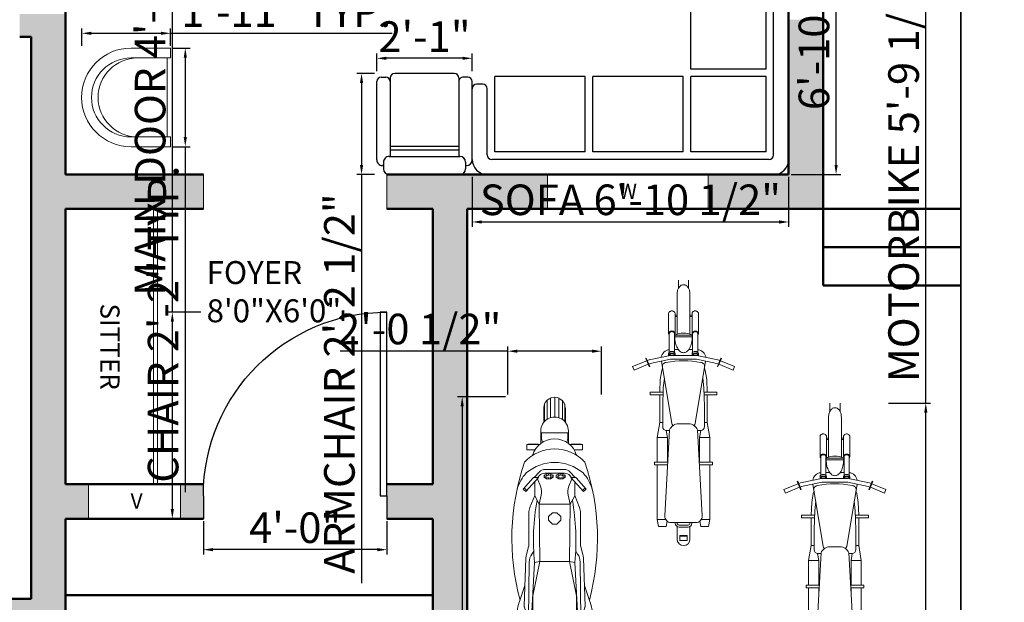
# Model space of a CAD drawing. Units: inches. Extents: x 3354 to 4308, y 1668 to 2317.
# Tile 4 of 11: x 3534 to 3792, y 1807 to 1960. Entities that reach past the tile are written whole.
import ezdxf

# ---------------------------------------------------------------- set-up
doc = ezdxf.new("R2010")
doc.units = ezdxf.units.IN
for name, color, linetype, lineweight in [('A-ANNO-DIMS', 2, 'Continuous', 18), ('A-ANNO-TEXT', 7, 'Continuous', 18), ('A-AREA-IDEN', 3, 'Continuous', 18), ('A-DOOR', 3, 'Continuous', 25), ('A-EQPM', 9, 'Continuous', 18), ('A-FURN', 8, 'Continuous', 18), ('A-GLAZ', 4, 'Continuous', 18), ('A-WALL', 7, 'Continuous', 50), ('A-WALL-PATT', 8, 'Continuous', 13), ('C-PROP', 1, 'Continuous', 35)]:
    doc.layers.add(name, color=color, linetype=linetype, lineweight=lineweight)
doc.layers.add('M40-KOLTUKSUNGERI', color=136, linetype='Continuous')
doc.layers.add('wood', color=26, linetype='Continuous')
doc.styles.get("Standard").update_dxf_attribs({"font": 'arial.ttf'})
doc.dimstyles.new('ISO-25', dxfattribs={"dimtxt": 8, "dimasz": 2.5, "dimexe": 1.25, "dimexo": 0.625, "dimtad": 1, "dimdec": 1, "dimlunit": 3, "dimtxsty": 'Standard', "dimcen": 2.5, "dimadec": 0, "dimazin": 0, "dimtfac": 1, "dimtdec": 1, "dimtmove": 0, "dimatfit": 3, "dimfxl": 1, "dimarcsym": 0})

# ---------------------------------------------------------------- blocks, each defined once
blk = doc.blocks.new('DOOR')
for p, q in [((0, 6), (0, 0)), ((48, 6), (48, 0))]:
    blk.add_line(p, q)
blk.add_lwpolyline([(0, 6), (0, 54), (1.75, 54), (1.75, 6)], close=True)
blk.add_arc((0, 6), 48, 0, 90)
blk = doc.blocks.new('12PSTG07')
at = {"color": 0, "linetype": 'ByBlock'}
for p, q in [((0, 15), (-12, 15)), ((0, 12), (0, 15)), ((-12, 12), (0, 12)), ((-1, -12), (-1, 12)), ((-12, -12), (0, -12)), ((0, -12), (0, -15)), ((0, -15), (-12, -15))]:
    blk.add_line(p, q, dxfattribs=at)
for centre, radius in [((-12, 0), 15), ((-12, 0), 12), ((-10, 0), 12)]:
    blk.add_arc(centre, radius, 90, 270, dxfattribs=at)
blk = doc.blocks.new('BIKE')
for p, q in [((34846.04, 15170.34), (34846.04, 15168.87)), ((34847.86, 15170.34), (34847.86, 15168.87)), ((34845.81, 15167.86), (34845.81, 15160.7)), ((34845.81, 15167.86), (34845.81, 15160.7)), ((34848.09, 15167.86), (34848.09, 15160.7)), ((34844.29, 15164.4), (34844.29, 15160.81)), ((34845.43, 15164.4), (34845.43, 15160.81)), ((34845.43, 15164.1), (34845.81, 15164.1)), ((34845.43, 15163.85), (34845.81, 15163.85)), ((34848.47, 15164.1), (34848.09, 15164.1)), ((34848.47, 15163.85), (34848.09, 15163.85)), ((34848.47, 15164.4), (34848.47, 15160.81)), ((34849.61, 15164.4), (34849.61, 15160.81)), ((34844.41, 15160.81), (34844.41, 15157.43)), ((34845.32, 15160.81), (34845.32, 15157.43)), ((34848.51, 15160.53), (34845.39, 15160.53)), ((34845.39, 15160.23), (34845.39, 15160.53)), ((34845.39, 15160.23), (34845.39, 15160.53)), ((34848.51, 15160.23), (34845.39, 15160.23)), ((34848.51, 15160.23), (34848.51, 15160.53)), ((34848.58, 15160.81), (34848.58, 15157.43)), ((34849.5, 15160.81), (34849.5, 15157.43)), ((34845.32, 15157.92), (34846.04, 15157.92)), ((34848.58, 15157.92), (34847.87, 15157.92)), ((34837.84, 15154.89), (34840.37, 15155.93)), ((34840.19, 15156.35), (34840.3, 15156.39)), ((34840.19, 15156.35), (34840.8, 15154.88)), ((34840.3, 15156.39), (34840.9, 15154.92)), ((34840.47, 15155.97), (34840.8, 15156.11)), ((34840.8, 15156.11), (34844.56, 15156.88)), ((34841, 15155.45), (34844.63, 15156.2)), ((34844.86, 15144.72), (34843.01, 15155.87)), ((34844.29, 15156.87), (34844.29, 15157.17)), ((34844.41, 15156.87), (34844.41, 15156.85)), ((34844.56, 15156.88), (34846.95, 15156.88)), ((34844.63, 15156.2), (34846.95, 15156.2)), ((34845.43, 15156.87), (34845.43, 15157.17)), ((34849.34, 15156.88), (34846.95, 15156.88)), ((34849.27, 15156.2), (34846.95, 15156.2)), ((34848.47, 15156.87), (34848.47, 15157.17)), ((34849.05, 15144.72), (34850.89, 15155.87)), ((34852.9, 15155.45), (34849.27, 15156.2)), ((34853.1, 15156.11), (34849.34, 15156.88)), ((34849.5, 15156.87), (34849.5, 15156.85)), ((34849.61, 15156.87), (34849.61, 15157.17)), ((34853.6, 15156.39), (34853, 15154.92)), ((34853.71, 15156.35), (34853.1, 15154.88)), ((34853.43, 15155.97), (34853.1, 15156.11)), ((34856.07, 15154.89), (34853.54, 15155.93)), ((34853.71, 15156.35), (34853.6, 15156.39)), ((34837.84, 15154.89), (34838.1, 15154.26)), ((34838.1, 15154.26), (34840.63, 15155.3)), ((34840.73, 15155.34), (34841, 15155.45)), ((34840.8, 15154.88), (34840.9, 15154.92)), ((34842.8, 15152.59), (34843.06, 15154.2)), ((34843.06, 15154.2), (34843.22, 15154.58)), ((34850.84, 15154.2), (34850.68, 15154.58)), ((34851.1, 15152.59), (34850.84, 15154.2)), ((34853.17, 15155.34), (34852.9, 15155.45)), ((34853.1, 15154.88), (34853, 15154.92)), ((34855.81, 15154.26), (34853.28, 15155.3)), ((34856.07, 15154.89), (34855.81, 15154.26)), ((34842.7, 15150.31), (34842.8, 15152.59)), ((34843.33, 15151.09), (34843.52, 15152.8)), ((34850.57, 15151.09), (34850.38, 15152.8)), ((34851.2, 15150.31), (34851.1, 15152.59)), ((34843.23, 15147.75), (34843.33, 15151.09)), ((34850.67, 15147.75), (34850.57, 15151.09)), ((34840.97, 15150.31), (34843.3, 15150.31)), ((34840.97, 15149.81), (34840.97, 15150.31)), ((34843.29, 15149.81), (34840.97, 15149.81)), ((34842.7, 15144.87), (34842.7, 15149.81)), ((34852.93, 15150.31), (34850.6, 15150.31)), ((34850.61, 15149.81), (34852.93, 15149.81)), ((34851.2, 15144.87), (34851.2, 15149.81)), ((34852.93, 15149.81), (34852.93, 15150.31)), ((34843.23, 15144.15), (34843.23, 15147.75)), ((34850.67, 15144.15), (34850.67, 15147.75)), ((34842.7, 15144.87), (34842.25, 15142.19)), ((34842.7, 15144.87), (34843.23, 15144.87)), ((34844.46, 15143.56), (34843.6, 15128.2)), ((34847.85, 15144.64), (34846.06, 15144.64)), ((34849.44, 15143.56), (34850.3, 15128.2)), ((34851.2, 15144.87), (34850.67, 15144.87)), ((34851.2, 15144.87), (34851.65, 15142.19)), ((34842.25, 15142.19), (34844.07, 15142.19)), ((34842.25, 15137.82), (34842.25, 15142.19)), ((34843.85, 15143.46), (34844.07, 15142.19)), ((34843.91, 15143.46), (34844.46, 15143.46)), ((34844.07, 15137.82), (34844.07, 15142.19)), ((34849.99, 15143.46), (34849.44, 15143.46)), ((34850.05, 15143.46), (34849.83, 15142.19)), ((34851.65, 15142.19), (34849.83, 15142.19)), ((34849.83, 15137.82), (34849.83, 15142.19)), ((34851.65, 15137.82), (34851.65, 15142.19)), ((34841.79, 15137.82), (34844.14, 15137.82)), ((34841.79, 15137.33), (34841.79, 15137.82)), ((34844.11, 15137.33), (34841.79, 15137.33)), ((34842.25, 15127.57), (34842.25, 15137.33)), ((34844.07, 15136.55), (34844.07, 15137.33)), ((34852.11, 15137.82), (34849.76, 15137.82)), ((34849.79, 15137.33), (34852.11, 15137.33)), ((34849.83, 15136.55), (34849.83, 15137.33)), ((34851.65, 15127.57), (34851.65, 15137.33)), ((34852.11, 15137.33), (34852.11, 15137.82)), ((34842.25, 15127.57), (34843.75, 15127.57)), ((34842.25, 15127.57), (34842.48, 15126.27)), ((34842.48, 15126.27), (34843.84, 15126.27)), ((34844.02, 15127.25), (34843.84, 15126.27)), ((34849.16, 15126.99), (34844.74, 15126.99)), ((34845.47, 15126.99), (34845.47, 15126.88)), ((34845.81, 15126.99), (34845.81, 15126.88)), ((34845.81, 15126.29), (34845.81, 15124.03)), ((34847.75, 15126.54), (34846.15, 15126.54)), ((34847.75, 15126.2), (34846.15, 15126.2)), ((34848.09, 15126.99), (34848.09, 15126.88)), ((34848.09, 15126.29), (34848.09, 15124.03)), ((34848.43, 15126.99), (34848.43, 15126.88)), ((34849.89, 15127.25), (34850.06, 15126.27)), ((34851.43, 15126.27), (34850.06, 15126.27)), ((34851.65, 15127.57), (34850.15, 15127.57)), ((34851.65, 15127.57), (34851.43, 15126.27)), ((34846.29, 15123.82), (34846.29, 15124.66)), ((34846.29, 15124.66), (34847.61, 15124.66)), ((34846.29, 15124.55), (34847.61, 15124.55)), ((34847.61, 15124.66), (34847.61, 15123.82)), ((34847.61, 15123.82), (34846.29, 15123.82))]:
    blk.add_line(p, q)
for points in [[(34845.81, 15167.86, -0.068977), (34845.9, 15168.53, -0.081012), (34846.15, 15169.05, -0.107014), (34846.54, 15169.42, -0.137239), (34846.95, 15169.53, -0.137239), (34847.36, 15169.42, -0.107014), (34847.76, 15169.05, -0.081012), (34848, 15168.53, -0.068977), (34848.09, 15167.86, -0.068977)], [(34845.43, 15164.4, 0.125099), (34845.39, 15164.56, 0.105827), (34845.27, 15164.71, 0.086577), (34845.09, 15164.8, 0.0766), (34844.86, 15164.84, 0.0766), (34844.64, 15164.8, 0.086577), (34844.46, 15164.71, 0.105827), (34844.33, 15164.56, 0.125099), (34844.29, 15164.4, 0.125099)], [(34848.47, 15164.4, -0.125099), (34848.51, 15164.56, -0.105827), (34848.64, 15164.71, -0.086577), (34848.82, 15164.8, -0.0766), (34849.04, 15164.84, -0.0766), (34849.26, 15164.8, -0.086577), (34849.44, 15164.71, -0.105827), (34849.57, 15164.56, -0.125099), (34849.61, 15164.4, -0.125099)], [(34845.32, 15160.55, 0.067261), (34845.39, 15160.65, 0.125099), (34845.43, 15160.81, 0.125099), (34845.39, 15160.97, 0.105827), (34845.27, 15161.12, 0.086577), (34845.09, 15161.21, 0.0766), (34844.86, 15161.25, 0.0766), (34844.64, 15161.21, 0.086577), (34844.46, 15161.12, 0.105827), (34844.33, 15160.97, 0.125099), (34844.29, 15160.81, 0.125099)], [(34845.32, 15160.81, 0.125099), (34845.29, 15160.92, 0.105827), (34845.2, 15161.03, 0.086577), (34845.05, 15161.1, 0.0766), (34844.86, 15161.13, 0.0766), (34844.67, 15161.1, 0.086577), (34844.53, 15161.03, 0.105827), (34844.43, 15160.92, 0.125099), (34844.41, 15160.81, 0.125099)], [(34848.58, 15160.55, -0.067261), (34848.51, 15160.65, -0.125099), (34848.47, 15160.81, -0.125099), (34848.51, 15160.97, -0.105827), (34848.64, 15161.12, -0.086577), (34848.82, 15161.21, -0.0766), (34849.04, 15161.25, -0.0766), (34849.26, 15161.21, -0.086577), (34849.44, 15161.12, -0.105827), (34849.57, 15160.97, -0.125099), (34849.61, 15160.81, -0.125099)], [(34848.58, 15160.81, -0.125099), (34848.61, 15160.92, -0.105827), (34848.71, 15161.03, -0.086577), (34848.85, 15161.1, -0.0766), (34849.04, 15161.13, -0.0766), (34849.23, 15161.1, -0.086577), (34849.37, 15161.03, -0.105827), (34849.47, 15160.92, -0.125099), (34849.5, 15160.81, -0.125099)], [(34844.29, 15160.81, 0.125099), (34844.33, 15160.65, 0.067261), (34844.41, 15160.55, 0.086577)], [(34846.95, 15157.37, -0.163989), (34846.41, 15157.55, -0.105862), (34845.85, 15158.21, -0.069323), (34845.52, 15159.08, -0.055531), (34845.39, 15160.23, -0.055531)], [(34848.51, 15160.23, -0.055531), (34848.38, 15159.08, -0.069323), (34848.06, 15158.21, -0.105862), (34847.49, 15157.55, -0.163989), (34846.95, 15157.37, -0.163989)], [(34849.61, 15160.81, -0.125099), (34849.57, 15160.65, -0.067261), (34849.5, 15160.55, -0.086577)], [(34845.43, 15157.17, 0.125099), (34845.39, 15157.33, 0.105827), (34845.27, 15157.48, 0.086577), (34845.09, 15157.57, 0.0766), (34844.86, 15157.6, 0.0766), (34844.64, 15157.57, 0.086577), (34844.46, 15157.48, 0.105827), (34844.33, 15157.33, 0.125099), (34844.29, 15157.17, 0.125099)], [(34848.47, 15157.17, -0.125099), (34848.51, 15157.33, -0.105827), (34848.64, 15157.48, -0.086577), (34848.82, 15157.57, -0.0766), (34849.04, 15157.6, -0.0766), (34849.26, 15157.57, -0.086577), (34849.44, 15157.48, -0.105827), (34849.57, 15157.33, -0.125099), (34849.61, 15157.17, -0.125099)], [(34845.43, 15156.88, 0.117252), (34845.39, 15157.03, 0.105827), (34845.27, 15157.18, 0.086577), (34845.09, 15157.27, 0.0766), (34844.86, 15157.31, 0.0766), (34844.64, 15157.27, 0.086577), (34844.46, 15157.18, 0.105827), (34844.33, 15157.03, 0.125099), (34844.29, 15156.87, 0.125099)], [(34844.29, 15156.87, 0.032819), (34844.3, 15156.83, 0.067261)], [(34845.32, 15156.88, 0.113202), (34845.29, 15156.98, 0.105827), (34845.2, 15157.09, 0.086577), (34845.05, 15157.16, 0.0766), (34844.86, 15157.19, 0.0766), (34844.67, 15157.16, 0.086577), (34844.53, 15157.09, 0.105827), (34844.43, 15156.98, 0.125099), (34844.41, 15156.87, 0.125099)], [(34848.47, 15156.88, -0.117252), (34848.51, 15157.03, -0.105827), (34848.64, 15157.18, -0.086577), (34848.82, 15157.27, -0.0766), (34849.04, 15157.31, -0.0766), (34849.26, 15157.27, -0.086577), (34849.44, 15157.18, -0.105827), (34849.57, 15157.03, -0.125099), (34849.61, 15156.87, -0.125099)], [(34848.58, 15156.88, -0.113202), (34848.61, 15156.98, -0.105827), (34848.71, 15157.09, -0.086577), (34848.85, 15157.16, -0.0766), (34849.04, 15157.19, -0.0766), (34849.23, 15157.16, -0.086577), (34849.37, 15157.09, -0.105827), (34849.47, 15156.98, -0.125099), (34849.5, 15156.87, -0.125099)], [(34849.61, 15156.87, -0.032819), (34849.61, 15156.83, -0.067261)]]:
    blk.add_lwpolyline(points, format="xyb")
for centre, radius, start, end in [((34846.95, 15157.24), 3.64, 64.5882, 115.4118), ((34844.55, 15156.32), 1.59, 95.2207, 171.678), ((34849.35, 15156.32), 1.59, 8.322, 84.7793), ((34846.95, 15140.12), 15.79, 78.7129, 101.2871), ((34843.86, 15154.92), 0.684, 90, 189.3898), ((34850.04, 15154.92), 0.684, 350.6102, 90), ((34843.91, 15144.15), 0.684, 180, 270), ((34846, 15143), 1.64, 88.1125, 159.9264), ((34845.53, 15144.83), 0.684, 189.3898, 226.4877), ((34847.9, 15143), 1.64, 20.0736, 91.8875), ((34848.37, 15144.83), 0.684, 313.5123, 350.6102), ((34849.99, 15144.15), 0.684, 270, 0), ((34844.74, 15128.13), 1.14, 176.7865, 270), ((34849.16, 15128.13), 1.14, 270, 3.2135), ((34846.15, 15126.88), 0.684, 180, 270), ((34846.15, 15126.88), 0.342, 180, 270), ((34847.75, 15126.88), 0.684, 270, 0), ((34847.75, 15126.88), 0.342, 270, 0), ((34846.95, 15124.03), 1.14, 180, 0)]:
    blk.add_arc(centre, radius, start, end)
blk = doc.blocks.new('1 bike')
for p, q in [((-13.2, 41.5), (-13.2, 35.26)), ((-12.29, 42.13), (-12.29, 35.26)), ((-11.19, 35.26), (-11.19, 42.36)), ((-10.09, 42.17), (-10.09, 35.26)), ((-9.19, 41.55), (-9.19, 35.26)), ((-14.01, 39.55), (-14.01, 35.26)), ((-13.81, 35.26), (-13.81, 40.5)), ((-8.57, 35.26), (-8.57, 40.59)), ((-8.38, 39.55), (-8.38, 35.26)), ((-17.37, 30.6), (-16.62, 34.32)), ((-14.57, 34.95), (-15.85, 34.95)), ((-7.36, 33.82), (-15.02, 33.82)), ((-14.78, 35.24), (-14.17, 34.43)), ((-14.78, 35.24), (-7.6, 35.24)), ((-8.21, 34.43), (-14.17, 34.43)), ((-7.6, 35.24), (-8.21, 34.43)), ((-7.81, 34.95), (-6.53, 34.95)), ((-5.01, 30.6), (-5.76, 34.32)), ((-21.27, 32.95), (-21.54, 32.62)), ((-21.54, 32.62), (-21.28, 21.37)), ((-18.78, 32.95), (-21.27, 32.95)), ((-18.78, 32.95), (-18.43, 32.54)), ((-18.43, 32.54), (-18.57, 30.5)), ((-18.18, 30.5), (-18.46, 32.12)), ((-16.53, 30.42), (-15.78, 33.23)), ((-5.85, 30.42), (-6.6, 33.23)), ((-4.2, 30.5), (-3.92, 32.12)), ((-3.61, 32.95), (-3.95, 32.54)), ((-3.95, 32.54), (-3.81, 30.5)), ((-3.61, 32.95), (-1.11, 32.95)), ((-1.11, 32.95), (-0.84, 32.62)), ((-0.84, 32.62), (-1.1, 21.37)), ((-20.57, 28.93), (-20.57, 30.49)), ((-20.57, 30.49), (-16.95, 30.49)), ((-16.95, 28.93), (-20.57, 28.93)), ((-20.22, 30.58), (-17.31, 30.58)), ((-18.58, 28.93), (-18.58, 23.76)), ((-17.89, 28.92), (-17.63, 27.46)), ((-17.5, 28.92), (-17.66, 26.86)), ((-17.37, 30.5), (-17.37, 30.6)), ((-16.53, 30.42), (-17.37, 30.55)), ((-17.37, 30.55), (-17.37, 30.5)), ((-16.95, 30.49), (-16.95, 28.93)), ((-16.04, 27.32), (-16.53, 30.42)), ((-5.85, 30.42), (-16.5, 30.42)), ((-6.34, 27.32), (-5.85, 30.42)), ((-5.85, 30.42), (-5.01, 30.55)), ((-5.43, 30.49), (-5.43, 28.93)), ((-1.81, 30.49), (-5.43, 30.49)), ((-5.43, 28.93), (-1.81, 28.93)), ((-2.16, 30.58), (-5.08, 30.58)), ((-5.01, 30.5), (-5.01, 30.6)), ((-5.01, 30.55), (-5.01, 30.5)), ((-4.88, 28.92), (-4.72, 26.86)), ((-4.49, 28.92), (-4.75, 27.46)), ((-3.8, 28.93), (-3.8, 23.76)), ((-1.81, 28.93), (-1.81, 30.49)), ((-19.32, 21.36), (-17.66, 26.86)), ((-19.19, 21.42), (-16.04, 27.32)), ((-16.04, 27.32), (-17.98, 21.16)), ((-16.17, 25.96), (-16.89, 22.88)), ((-15.14, 27.32), (-16.17, 25.96)), ((-16.04, 27.32), (-16.08, 26.1)), ((-16.01, 27.32), (-6.34, 27.32)), ((-15.14, 24.28), (-15.14, 27.32)), ((-7.24, 27.32), (-6.21, 25.96)), ((-7.24, 24.28), (-7.24, 27.32)), ((-6.34, 27.32), (-6.31, 26.1)), ((-6.34, 27.32), (-4.4, 21.16)), ((-3.2, 21.42), (-6.34, 27.32)), ((-6.21, 25.96), (-5.5, 22.88)), ((-3.07, 21.36), (-4.72, 26.86)), ((-16.17, 21.85), (-15.14, 24.28)), ((-7.24, 24.28), (-15.11, 24.28)), ((-6.21, 21.85), (-7.24, 24.28)), ((-17.84, 6.18), (-18.02, 20.91)), ((-16.89, 22.88), (-17.14, 19.13)), ((-16.89, 19.03), (-16.17, 21.85)), ((-5.5, 19.03), (-6.21, 21.85)), ((-5.5, 22.88), (-5.24, 19.13)), ((-4.54, 6.18), (-4.37, 20.91)), ((-19.11, 17.99), (-18.54, 19.9)), ((-19.09, 20.53), (-18, 19.28)), ((-17.14, 19.13), (-16.46, 6.25)), ((-16.92, 15.02), (-16.89, 19.03)), ((-5.24, 19.13), (-5.92, 6.25)), ((-5.46, 15.02), (-5.5, 19.03)), ((-3.3, 20.53), (-4.39, 19.28)), ((-3.27, 17.99), (-3.84, 19.9)), ((-18.96, 12.28), (-20.45, 16.7)), ((-18.71, 5.16), (-19.15, 17.74)), ((-3.67, 5.16), (-3.24, 17.74)), ((-3.42, 12.28), (-1.93, 16.7)), ((-15.04, 6), (-16.92, 15.02)), ((-7.34, 6), (-5.46, 15.02)), ((-15.04, 6), (-16.46, 6.25)), ((-15.04, 6), (-16.46, 6.25)), ((-15.27, -8.98), (-15.04, 6)), ((-15.01, 6), (-7.34, 6)), ((-15.01, 6), (-7.34, 6)), ((-7.34, 6), (-5.92, 6.25)), ((-7.34, 6), (-5.92, 6.25)), ((-7.11, -8.98), (-7.34, 6)), ((-18.09, 2.47), (-18.58, 4.26)), ((-17.19, 4.06), (-16.68, 3.28)), ((-5.19, 4.06), (-5.71, 3.28)), ((-4.3, 2.47), (-3.81, 4.26)), ((-17.95, -6.66), (-17.95, 1.43)), ((-4.43, -6.66), (-4.43, 1.43)), ((-11.77, -3.74), (-12.84, -4.75)), ((-12.84, -4.75), (-12.84, -5.75)), ((-11.77, -3.74), (-10.61, -3.74)), ((-10.61, -3.74), (-9.54, -4.75)), ((-9.54, -4.75), (-9.54, -5.75)), ((-12.84, -5.75), (-11.77, -6.72)), ((-10.61, -6.72), (-11.77, -6.72)), ((-9.54, -5.75), (-10.61, -6.72)), ((-16.42, -11.25), (-17.67, -8.11)), ((-15.27, -8.98), (-16.42, -11.15)), ((-14.73, -11.31), (-15.27, -8.98)), ((-7.11, -8.98), (-15.24, -8.98)), ((-7.65, -11.31), (-7.11, -8.98)), ((-7.11, -8.98), (-5.96, -11.15)), ((-5.96, -11.25), (-4.71, -8.11)), ((-18.7, -12.25), (-19.45, -12.92)), ((-18.44, -12.54), (-19.19, -13.22)), ((-15.4, -15.97), (-18.7, -12.25)), ((-16.42, -11.15), (-16.42, -14.82)), ((-6.99, -15.97), (-3.68, -12.25)), ((-5.96, -11.15), (-5.96, -14.82)), ((-3.94, -12.54), (-3.19, -13.22)), ((-3.68, -12.25), (-2.93, -12.92)), ((-19.45, -12.92), (-16.84, -15.84)), ((-15.69, -15.57), (-14.92, -13.66)), ((-6.69, -15.57), (-7.46, -13.66)), ((-2.93, -12.92), (-5.54, -15.84)), ((-16.55, -15.97), (-15.4, -15.97)), ((-16.51, -15.99), (-15.16, -17.42)), ((-15.17, -16.45), (-15.61, -15.99)), ((-13.97, -16), (-13.29, -15.62)), ((-13.97, -16.52), (-13.97, -16)), ((-13.29, -16.91), (-13.97, -16.52)), ((-13.29, -16.1), (-13.75, -16.04)), ((-13.75, -16.36), (-13.29, -16.26)), ((-13.74, -17.07), (-8.65, -17.07)), ((-13.39, -15.74), (-13.1, -15.97)), ((-13.1, -16.42), (-13.39, -16.62)), ((-12.29, -15.62), (-13.29, -15.62)), ((-12.29, -16.91), (-13.29, -16.91)), ((-12.78, -15.91), (-12.78, -15.65)), ((-12.78, -16.49), (-12.78, -16.72)), ((-12.19, -15.74), (-12.45, -15.97)), ((-12.45, -16.42), (-12.19, -16.62)), ((-12.29, -15.62), (-11.58, -16)), ((-12.29, -16.91), (-11.58, -16.52)), ((-11.81, -16.04), (-12.26, -16.1)), ((-12.26, -16.26), (-11.81, -16.36)), ((-11.58, -16.52), (-11.58, -16)), ((-10.09, -15.62), (-10.8, -16)), ((-10.8, -16.52), (-10.8, -16)), ((-10.09, -16.91), (-10.8, -16.52)), ((-10.58, -16.04), (-10.12, -16.1)), ((-10.12, -16.26), (-10.58, -16.36)), ((-10.19, -15.74), (-9.93, -15.97)), ((-9.93, -16.42), (-10.19, -16.62)), ((-10.09, -15.62), (-9.09, -15.62)), ((-10.09, -16.91), (-9.09, -16.91)), ((-9.61, -15.91), (-9.61, -15.65)), ((-9.61, -16.49), (-9.61, -16.72)), ((-8.99, -15.74), (-9.28, -15.97)), ((-9.28, -16.42), (-8.99, -16.62)), ((-8.41, -16), (-9.09, -15.62)), ((-9.09, -16.1), (-8.64, -16.04)), ((-8.64, -16.36), (-9.09, -16.26)), ((-9.09, -16.91), (-8.41, -16.52)), ((-8.41, -16.52), (-8.41, -16)), ((-5.87, -15.99), (-7.22, -17.42)), ((-7.21, -16.45), (-6.77, -15.99)), ((-5.83, -15.97), (-6.99, -15.97)), ((-8.65, -18.04), (-13.73, -18.04)), ((-18.47, -24.58), (-18.47, -23.15)), ((-18.47, -23.15), (-16.35, -23.15)), ((-3.91, -23.15), (-6.03, -23.15)), ((-3.91, -24.58), (-3.91, -23.15)), ((-15.14, -24.58), (-18.47, -24.58)), ((-15.49, -24.67), (-18.15, -24.67)), ((-14.79, -24.85), (-14.79, -28.11)), ((-14.34, -25.16), (-14.62, -26.07)), ((-8.04, -25.18), (-7.76, -26.07)), ((-7.56, -24.85), (-7.56, -28.11)), ((-7.24, -24.58), (-3.91, -24.58)), ((-6.89, -24.67), (-4.24, -24.67)), ((-14.62, -26.07), (-14.62, -27.65)), ((-7.76, -27.65), (-14.62, -27.65)), ((-7.76, -26.07), (-7.76, -27.65)), ((-14.01, -30.38), (-14.01, -34.12)), ((-13.81, -35.22), (-13.81, -30.6)), ((-8.57, -35.22), (-8.57, -30.64)), ((-8.38, -30.42), (-8.38, -34.12)), ((-13.2, -31.13), (-13.2, -36.13)), ((-12.29, -36.74), (-12.29, -31.57)), ((-11.19, -31.75), (-11.19, -36.94)), ((-10.09, -36.74), (-10.09, -31.58)), ((-9.19, -31.15), (-9.19, -36.13))]:
    blk.add_line(p, q)
for centre, radius, start, end in [((-15.85, 34.16), 0.787, 90, 168.6493), ((-15.02, 33.03), 0.787, 90, 165.0682), ((-7.36, 33.03), 0.787, 14.9318, 90), ((-6.53, 34.16), 0.787, 11.3507, 90), ((-5.53, 21.74), 15.75, 181.3575, 198.6942), ((-18.56, 21.13), 0.787, 163.2719, 220.9137), ((-18.49, 21.05), 0.787, 151.9424, 220.9137), ((-17.23, 20.92), 0.787, 162.5452, 180.6944), ((-5.15, 20.92), 0.787, 359.3056, 17.4548), ((-3.89, 21.05), 0.787, 319.0863, 28.0576), ((-3.82, 21.13), 0.787, 319.0863, 16.7281), ((-16.85, 21.74), 15.75, 341.3058, 358.6425), ((39.63, 0), 62.01, 164.9421, 198.7675), ((-18.36, 17.77), 0.787, 163.359, 181.9702), ((-62.01, 0), 62.01, 341.2325, 15.0579), ((-4.02, 17.77), 0.787, 358.0298, 16.641), ((-14.78, 5.3), 3.94, 181.9702, 195.2875), ((-13.9, 6.23), 3.94, 180.6944, 213.3274), ((43.19, 0.53), 59.93, 174.5142, 190.1132), ((-65.57, 0.53), 59.93, 349.8868, 5.4858), ((-8.48, 6.23), 3.94, 326.6726, 359.3056), ((-7.6, 5.3), 3.94, 344.7125, 358.0298), ((-21.88, 1.43), 3.94, 0, 15.2875), ((-0.5, 1.43), 3.94, 164.7125, 180), ((-14.01, -6.66), 3.94, 180, 201.6868), ((-8.37, -6.66), 3.94, 338.3132, 0), ((-18.57, -12.19), 3.94, 338.094, 12.9179), ((-3.81, -12.19), 3.94, 167.0821, 201.906), ((-9.61, -9.24), 11.99, 197.8857, 221.2009), ((-12.77, -9.24), 11.99, 318.7991, 342.1143), ((-11.17, -8.43), 11.44, 229.5475, 310.4525), ((-16.55, -15.58), 0.394, 221.8676, 270), ((-13.74, -15.1), 1.97, 223.2382, 270), ((-13.73, -16.07), 1.97, 223.2382, 270), ((-8.65, -15.1), 1.97, 270, 316.7618), ((-8.65, -16.07), 1.97, 270, 316.7618), ((-5.83, -15.58), 0.394, 270, 318.1324), ((-11.17, -12.72), 10.69, 222.5562, 317.4438), ((-11.17, -20.07), 6, 196.0578, 343.9425), ((-11.17, -28.13), 3.61, 179.6687, 0.3313), ((-11.17, -34.14), 2.8, 179.6687, 0.3313)]:
    blk.add_arc(centre, radius, start, end)
blk = doc.blocks.new('sofa 1')
at = {"layer": 'M40-KOLTUKSUNGERI'}
for p, q in [((72.87, 57.09), (54.36, 57.09)), ((53.18, 54.33), (53.18, 55.91)), ((71.69, 53.15), (54.36, 53.15)), ((72.87, -20.47), (72.87, 51.97)), ((76.8, -21.65), (76.8, 53.15)), ((51.21, 27.56), (51.21, 51.18)), ((70.9, 51.18), (51.21, 51.18)), ((70.9, 27.56), (70.9, 51.18)), ((70.9, 27.56), (51.21, 27.56)), ((51.21, 1.97), (51.21, 25.59)), ((70.9, 25.59), (51.21, 25.59)), ((70.9, 1.97), (70.9, 25.59)), ((0, -19.69), (0, 0)), ((0, -19.69), (0, 0)), ((23.62, 0), (0, 0)), ((23.62, -19.69), (23.62, 0)), ((25.59, -19.69), (25.59, 0)), ((49.21, 0), (25.59, 0)), ((49.21, -19.69), (49.21, 0)), ((70.9, 1.97), (51.21, 1.97)), ((70.9, 0), (51.21, 0)), ((51.21, -19.69), (51.21, 0)), ((70.9, -19.69), (70.9, 0)), ((-3.15, -1.97), (-4.72, -1.97)), ((-5.91, -21.65), (-5.91, -3.15)), ((-1.97, -20.47), (-1.97, -3.15)), ((23.62, -19.69), (0, -19.69)), ((49.21, -19.69), (25.59, -19.69)), ((70.9, -19.69), (51.21, -19.69)), ((71.69, -21.65), (-0.79, -21.65)), ((72.87, -25.59), (-1.97, -25.59))]:
    blk.add_line(p, q, dxfattribs=at)
for centre, radius, start, end in [((54.36, 55.91), 1.18, 90, 180), ((72.87, 53.15), 3.94, 0, 90), ((54.36, 54.33), 1.18, 180, 270), ((71.69, 51.97), 1.18, 0, 90), ((-4.72, -3.15), 1.18, 90, 180), ((-3.15, -3.15), 1.18, 0, 90), ((-0.79, -20.47), 1.18, 180, 270), ((71.69, -20.47), 1.18, 270, 0), ((-1.97, -21.65), 3.94, 180, 270), ((72.87, -21.65), 3.94, 270, 0)]:
    blk.add_arc(centre, radius, start, end, dxfattribs=at)
blk = doc.blocks.new('A$C38B70996')
at = {"layer": 'wood'}
for p, q in [((0.11, 0.9), (0.74, 0.9)), ((0.06, 0.82), (0.05, 0.82)), ((0.06, 0.79), (0.06, 0.85)), ((0.79, 0.79), (0.79, 0.85)), ((0.79, 0.82), (0.8, 0.82)), ((0, 0.77), (0, 0.073)), ((0.74, 0.74), (0.11, 0.74)), ((0.12, 0.04), (0.12, 0.74)), ((0.73, 0.04), (0.73, 0.74)), ((0.85, 0.77), (0.85, 0.073)), ((0.73, 0.68), (0.12, 0.68)), ((0.73, 0.647), (0.12, 0.647)), ((0.04, 0.033), (0.08, 0.033)), ((0.16, 0), (0.69, 0)), ((0.81, 0.033), (0.77, 0.033))]:
    blk.add_line(p, q, dxfattribs=at)
for centre, radius, start, end in [((0.11, 0.85), 0.05, 90, 180), ((0.74, 0.85), 0.05, 0, 90), ((0.05, 0.77), 0.05, 90, 180), ((0.11, 0.79), 0.05, 180, 270), ((0.74, 0.79), 0.05, 270, 0), ((0.8, 0.77), 0.05, 360, 90), ((0.04, 0.073), 0.04, 180, 270), ((0.08, 0.073), 0.04, 270, 0), ((0.16, 0.04), 0.04, 180, 270), ((0.69, 0.04), 0.04, 270, 360), ((0.77, 0.073), 0.04, 180, 270), ((0.81, 0.073), 0.04, 270, 360)]:
    blk.add_arc(centre, radius, start, end, dxfattribs=at)
blk = doc.blocks.new('*D52')
at = {"layer": 'A-ANNO-DIMS', "color": 0, "lineweight": -2, "transparency": 16777216}
for p, q in [((3574.32, 1952.36), (3578.81, 1952.36)), ((3577.56, 1949.86), (3577.56, 1929.07)), ((3574.32, 1926.57), (3578.81, 1926.57)), ((3577.56, 1926.57), (3577.56, 1836.27))]:
    blk.add_line(p, q, dxfattribs=at)
at = {"layer": 'A-ANNO-DIMS', "color": 0, "transparency": 16777216}
for points in [[(3577.15, 1949.86), (3577.98, 1949.86), (3577.56, 1952.36)], [(3577.15, 1929.07), (3577.98, 1929.07), (3577.56, 1926.57)]]:
    blk.add_solid(points, dxfattribs=at)
at = {"layer": 'Defpoints', "color": 0, "transparency": 16777216}
for p in [(3573.69, 1952.36), (3573.69, 1926.57), (3577.56, 1926.57)]:
    blk.add_point(p, dxfattribs=at)
at = {"layer": 'A-ANNO-DIMS', "color": 0, "transparency": 16777216, "insert": (3572.8, 1880.17), "char_height": 8, "attachment_point": 5, "rotation": 90}
blk.add_mtext('CHAIR 2\'-2" TYP.', dxfattribs=at)
blk = doc.blocks.new('*D53')
at = {"layer": 'A-ANNO-DIMS', "color": 0, "lineweight": -2, "transparency": 16777216}
for p, q in [((3550.48, 1952.98), (3550.48, 1957.48)), ((3552.98, 1956.23), (3571.19, 1956.23)), ((3573.69, 1952.98), (3573.69, 1957.48)), ((3573.69, 1956.23), (3631.67, 1956.23))]:
    blk.add_line(p, q, dxfattribs=at)
at = {"layer": 'A-ANNO-DIMS', "color": 0, "transparency": 16777216}
for points in [[(3552.98, 1956.64), (3552.98, 1955.81), (3550.48, 1956.23)], [(3571.19, 1956.64), (3571.19, 1955.81), (3573.69, 1956.23)]]:
    blk.add_solid(points, dxfattribs=at)
at = {"layer": 'Defpoints', "color": 0, "transparency": 16777216}
for p in [(3573.69, 1956.23), (3550.48, 1952.36), (3573.69, 1952.36)]:
    blk.add_point(p, dxfattribs=at)
at = {"layer": 'A-ANNO-DIMS', "color": 0, "transparency": 16777216, "insert": (3603.93, 1960.87), "char_height": 8, "attachment_point": 5}
blk.add_mtext('1\'-11" TYP.', dxfattribs=at)
blk = doc.blocks.new('*D56')
at = {"layer": 'A-ANNO-DIMS', "color": 0, "lineweight": -2, "transparency": 16777216}
for p, q in [((3626.98, 1945.73), (3622.39, 1945.73)), ((3623.64, 1943.23), (3623.64, 1921.8)), ((3626.98, 1919.3), (3622.39, 1919.3)), ((3623.64, 1919.3), (3623.64, 1812.46))]:
    blk.add_line(p, q, dxfattribs=at)
at = {"layer": 'A-ANNO-DIMS', "color": 0, "transparency": 16777216}
for points in [[(3623.22, 1943.23), (3624.06, 1943.23), (3623.64, 1945.73)], [(3623.22, 1921.8), (3624.06, 1921.8), (3623.64, 1919.3)]]:
    blk.add_solid(points, dxfattribs=at)
at = {"layer": 'Defpoints', "color": 0, "transparency": 16777216}
for p in [(3627.61, 1945.73), (3623.64, 1919.3), (3627.61, 1919.3)]:
    blk.add_point(p, dxfattribs=at)
at = {"layer": 'A-ANNO-DIMS', "color": 0, "transparency": 16777216, "insert": (3618.88, 1864.63), "char_height": 8, "attachment_point": 5, "rotation": 90}
blk.add_mtext('ARMCHAIR 2\'-2 1/2"', dxfattribs=at)
blk = doc.blocks.new('*D57')
at = {"layer": 'A-ANNO-DIMS', "color": 0, "lineweight": -2, "transparency": 16777216}
for p, q in [((3627.61, 1946.35), (3627.61, 1950.94)), ((3652.57, 1946.35), (3652.57, 1950.94)), ((3650.07, 1949.69), (3630.11, 1949.69))]:
    blk.add_line(p, q, dxfattribs=at)
at = {"layer": 'A-ANNO-DIMS', "color": 0, "transparency": 16777216}
for points in [[(3630.11, 1950.11), (3630.11, 1949.28), (3627.61, 1949.69)], [(3650.07, 1950.11), (3650.07, 1949.28), (3652.57, 1949.69)]]:
    blk.add_solid(points, dxfattribs=at)
at = {"layer": 'Defpoints', "color": 0, "transparency": 16777216}
for p in [(3627.61, 1949.69), (3627.61, 1945.73), (3652.57, 1945.73)]:
    blk.add_point(p, dxfattribs=at)
at = {"layer": 'A-ANNO-DIMS', "color": 0, "transparency": 16777216, "insert": (3640.09, 1954.33), "char_height": 8, "attachment_point": 5}
blk.add_mtext('2\'-1"', dxfattribs=at)
blk = doc.blocks.new('*D70')
at = {"layer": 'A-ANNO-DIMS', "color": 0, "lineweight": -2, "transparency": 16777216}
for p, q in [((3771.12, 1859.52), (3771.12, 2000.47)), ((3761.34, 1859.52), (3772.37, 1859.52)), ((3771.12, 1792.61), (3771.12, 1857.02)), ((3761.34, 1790.11), (3772.37, 1790.11))]:
    blk.add_line(p, q, dxfattribs=at)
at = {"layer": 'A-ANNO-DIMS', "color": 0, "transparency": 16777216}
for points in [[(3770.71, 1857.02), (3771.54, 1857.02), (3771.12, 1859.52)], [(3770.71, 1792.61), (3771.54, 1792.61), (3771.12, 1790.11)]]:
    blk.add_solid(points, dxfattribs=at)
at = {"layer": 'Defpoints', "color": 0, "transparency": 16777216}
for p in [(3760.71, 1859.52), (3771.12, 1859.52), (3760.71, 1790.11)]:
    blk.add_point(p, dxfattribs=at)
at = {"layer": 'A-ANNO-DIMS', "color": 0, "transparency": 16777216, "insert": (3766.36, 1931.24), "char_height": 8, "attachment_point": 5, "rotation": 90}
blk.add_mtext('MOTORBIKE 5\'-9 1/2" TYP.', dxfattribs=at)
blk = doc.blocks.new('*D72')
at = {"layer": 'A-ANNO-DIMS', "color": 0, "lineweight": -2, "transparency": 16777216}
for p, q in [((3661.24, 1861.18), (3648.7, 1861.18)), ((3649.95, 1858.68), (3649.95, 1784.26)), ((3661.24, 1781.76), (3648.7, 1781.76)), ((3649.95, 1781.76), (3649.95, 1668.3))]:
    blk.add_line(p, q, dxfattribs=at)
at = {"layer": 'A-ANNO-DIMS', "color": 0, "transparency": 16777216}
for points in [[(3649.53, 1858.68), (3650.36, 1858.68), (3649.95, 1861.18)], [(3649.53, 1784.26), (3650.36, 1784.26), (3649.95, 1781.76)]]:
    blk.add_solid(points, dxfattribs=at)
at = {"layer": 'Defpoints', "color": 0, "transparency": 16777216}
for p in [(3661.86, 1861.18), (3649.95, 1781.76), (3661.86, 1781.76)]:
    blk.add_point(p, dxfattribs=at)
at = {"layer": 'A-ANNO-DIMS', "color": 0, "transparency": 16777216, "insert": (3645.18, 1723.78), "char_height": 8, "attachment_point": 5, "rotation": 90}
blk.add_mtext('MOTORBIKE 6\'-7 1/2"', dxfattribs=at)
blk = doc.blocks.new('*D73')
at = {"layer": 'A-ANNO-DIMS', "color": 0, "lineweight": -2, "transparency": 16777216}
for p, q in [((3661.86, 1861.81), (3661.86, 1874.35)), ((3686.37, 1861.81), (3686.37, 1874.35)), ((3661.86, 1873.1), (3618.07, 1873.1)), ((3683.87, 1873.1), (3664.36, 1873.1))]:
    blk.add_line(p, q, dxfattribs=at)
at = {"layer": 'A-ANNO-DIMS', "color": 0, "transparency": 16777216}
for points in [[(3664.36, 1873.51), (3664.36, 1872.68), (3661.86, 1873.1)], [(3683.87, 1873.51), (3683.87, 1872.68), (3686.37, 1873.1)]]:
    blk.add_solid(points, dxfattribs=at)
at = {"layer": 'Defpoints', "color": 0, "transparency": 16777216}
for p in [(3661.86, 1873.1), (3661.86, 1861.18), (3686.37, 1861.18)]:
    blk.add_point(p, dxfattribs=at)
at = {"layer": 'A-ANNO-DIMS', "color": 0, "transparency": 16777216, "insert": (3638.71, 1877.86), "char_height": 8, "attachment_point": 5}
blk.add_mtext('2\'-0 1/2"', dxfattribs=at)
blk = doc.blocks.new('*D74')
at = {"layer": 'A-ANNO-DIMS', "color": 0, "lineweight": -2, "transparency": 16777216}
for p, q in [((3574.18, 1883.3), (3574.18, 1975.62)), ((3581.65, 1883.3), (3572.93, 1883.3)), ((3574.18, 1831.8), (3574.18, 1880.8)), ((3581.65, 1829.3), (3572.93, 1829.3))]:
    blk.add_line(p, q, dxfattribs=at)
at = {"layer": 'A-ANNO-DIMS', "color": 0, "transparency": 16777216}
for points in [[(3573.76, 1880.8), (3574.59, 1880.8), (3574.18, 1883.3)], [(3573.76, 1831.8), (3574.59, 1831.8), (3574.18, 1829.3)]]:
    blk.add_solid(points, dxfattribs=at)
at = {"layer": 'Defpoints', "color": 0, "transparency": 16777216}
for p in [(3574.18, 1883.3), (3582.28, 1883.3), (3582.28, 1829.3)]:
    blk.add_point(p, dxfattribs=at)
at = {"layer": 'A-ANNO-DIMS', "color": 0, "transparency": 16777216, "insert": (3569.41, 1930.71), "char_height": 8, "attachment_point": 5, "rotation": 90}
blk.add_mtext('MAIN DOOR 4\'-6"', dxfattribs=at)
blk = doc.blocks.new('*D75')
at = {"layer": 'A-ANNO-DIMS', "color": 0, "lineweight": -2, "transparency": 16777216}
for p, q in [((3582.28, 1828.67), (3582.28, 1819.95)), ((3630.28, 1828.67), (3630.28, 1819.95)), ((3627.78, 1821.2), (3584.78, 1821.2))]:
    blk.add_line(p, q, dxfattribs=at)
at = {"layer": 'A-ANNO-DIMS', "color": 0, "transparency": 16777216}
for points in [[(3584.78, 1821.61), (3584.78, 1820.78), (3582.28, 1821.2)], [(3627.78, 1821.61), (3627.78, 1820.78), (3630.28, 1821.2)]]:
    blk.add_solid(points, dxfattribs=at)
at = {"layer": 'Defpoints', "color": 0, "transparency": 16777216}
for p in [(3582.28, 1829.3), (3630.28, 1829.3), (3582.28, 1821.2)]:
    blk.add_point(p, dxfattribs=at)
at = {"layer": 'A-ANNO-DIMS', "color": 0, "transparency": 16777216, "insert": (3606.28, 1825.91), "char_height": 8, "attachment_point": 5}
blk.add_mtext('4\'-0"', dxfattribs=at)
blk = doc.blocks.new('*D86')
at = {"layer": 'A-ANNO-DIMS', "color": 0, "lineweight": -2, "transparency": 16777216}
for p, q in [((3652.57, 1918.67), (3652.57, 1905.64)), ((3735.28, 1918.67), (3735.28, 1905.64)), ((3655.07, 1906.89), (3732.78, 1906.89))]:
    blk.add_line(p, q, dxfattribs=at)
at = {"layer": 'A-ANNO-DIMS', "color": 0, "transparency": 16777216}
for points in [[(3655.07, 1907.31), (3655.07, 1906.47), (3652.57, 1906.89)], [(3732.78, 1907.31), (3732.78, 1906.47), (3735.28, 1906.89)]]:
    blk.add_solid(points, dxfattribs=at)
at = {"layer": 'Defpoints', "color": 0, "transparency": 16777216}
for p in [(3652.57, 1919.3), (3735.28, 1919.3), (3735.28, 1906.89)]:
    blk.add_point(p, dxfattribs=at)
at = {"layer": 'A-ANNO-DIMS', "color": 0, "transparency": 16777216, "insert": (3693.92, 1911.65), "char_height": 8, "attachment_point": 5}
blk.add_mtext('SOFA 6\'-10 1/2"', dxfattribs=at)
blk = doc.blocks.new('*D87')
at = {"layer": 'A-ANNO-DIMS', "color": 0, "lineweight": -2, "transparency": 16777216}
for p, q in [((3735.9, 2001.97), (3748.93, 2001.97)), ((3747.68, 1921.8), (3747.68, 1999.47)), ((3735.9, 1919.3), (3748.93, 1919.3))]:
    blk.add_line(p, q, dxfattribs=at)
at = {"layer": 'A-ANNO-DIMS', "color": 0, "transparency": 16777216}
for points in [[(3747.27, 1999.47), (3748.1, 1999.47), (3747.68, 2001.97)], [(3747.27, 1921.8), (3748.1, 1921.8), (3747.68, 1919.3)]]:
    blk.add_solid(points, dxfattribs=at)
at = {"layer": 'Defpoints', "color": 0, "transparency": 16777216}
for p in [(3735.28, 2001.97), (3747.68, 2001.97), (3735.28, 1919.3)]:
    blk.add_point(p, dxfattribs=at)
at = {"layer": 'A-ANNO-DIMS', "color": 0, "transparency": 16777216, "insert": (3742.92, 1960.64), "char_height": 8, "attachment_point": 5, "rotation": 90}
blk.add_mtext('6\'-10 1/2"', dxfattribs=at)

msp = doc.modelspace()

# ---------------------------------------------------------------- hatches: boundary and pattern name
at = {"layer": 'A-WALL-PATT', "transparency": 33554687}
h = msp.add_hatch(color=256, dxfattribs=at)
h.dxf.hatch_style = 1
h.paths.add_polyline_path([(3546.28, 1829.3), (3552.28, 1829.3), (3552.28, 1838.3), (3546.28, 1838.3), (3546.28, 1910.3), (3582.28, 1910.3), (3582.28, 1919.3), (3546.28, 1919.3), (3546.28, 1961.3), (3534.28, 1961.3), (3534.28, 1955.3), (3537.28, 1955.3), (3537.28, 1808.3), (3516.28, 1808.3), (3516.28, 1799.3), (3546.28, 1799.3)])
h.paths.add_polyline_path([(3672.28, 1919.3), (3656.51, 1919.3), (3630.28, 1919.3), (3630.28, 1910.3), (3642.28, 1910.3), (3642.28, 1838.3), (3630.28, 1838.3), (3630.28, 1835.3), (3630.28, 1829.3), (3642.28, 1829.3), (3642.28, 1799.3), (3651.28, 1799.3), (3651.28, 1910.3), (3672.28, 1910.3)])
h.paths.add_polyline_path([(3744.28, 1959.8), (3735.28, 1959.8), (3735.28, 1923.23), (3735.28, 1919.3), (3714.28, 1919.3), (3714.28, 1910.3), (3744.28, 1910.3)])
h.paths.add_polyline_path([(3744.28, 2072.3), (3735.28, 2072.3), (3735.28, 2031.8), (3744.28, 2031.8)])
h.paths.add_polyline_path([(3744.28, 2150.3), (3735.28, 2150.3), (3735.28, 2108.3), (3744.28, 2108.3)])
h.paths.add_polyline_path([(3744.28, 2258.3), (3705.28, 2258.3), (3705.28, 2249.3), (3735.28, 2249.3), (3735.28, 2210.3), (3744.28, 2210.3)])
h.paths.add_polyline_path([(3633.28, 2258.3), (3583.78, 2258.3), (3583.78, 2249.3), (3588.24, 2249.3), (3597.28, 2249.3), (3597.28, 2165.3), (3594.28, 2165.3), (3594.28, 2159.3), (3597.28, 2159.3), (3597.28, 2117.3), (3594.28, 2117.3), (3594.28, 2111.3), (3603.28, 2111.3), (3603.28, 2249.3), (3633.28, 2249.3)])
h.paths.add_polyline_path([(3559.78, 2258.3), (3492.28, 2258.3), (3492.28, 2249.3), (3537.28, 2249.3), (3537.28, 2117.3), (3534.28, 2117.3), (3534.28, 2111.3), (3564.28, 2111.3), (3564.28, 2117.3), (3546.28, 2117.3), (3546.28, 2159.3), (3564.28, 2159.3), (3564.28, 2165.3), (3546.28, 2165.3), (3546.28, 2249.3), (3559.78, 2249.3)])
h.paths.add_polyline_path([(3450.28, 2258.3), (3396.28, 2258.3), (3396.28, 1799.3), (3474.28, 1799.3), (3474.28, 1808.3), (3405.28, 1808.3), (3405.28, 1955.3), (3498.28, 1955.3), (3498.28, 1961.3), (3405.28, 1961.3), (3405.28, 2111.3), (3498.28, 2111.3), (3498.28, 2117.3), (3405.28, 2117.3), (3405.28, 2249.3), (3450.28, 2249.3)])
h.paths.add_polyline_path([(3582.28, 1838.3), (3576.28, 1838.3), (3576.28, 1829.3), (3582.28, 1829.3)], flags=17)

# ---------------------------------------------------------------- linework, layer by layer
at = {"layer": 'A-FURN'}
for p, q in [((3569.28, 1910.3), (3569.28, 1838.3)), ((3570.28, 1910.3), (3570.28, 1838.3))]:
    msp.add_line(p, q, dxfattribs=at)
at = {"layer": 'A-GLAZ'}
for p, q in [((3582.28, 1919.3), (3582.28, 1910.3)), ((3630.28, 1919.3), (3630.28, 1910.3)), ((3672.28, 1919.3), (3672.28, 1910.3)), ((3714.28, 1919.3), (3714.28, 1910.3)), ((3552.28, 1838.3), (3552.28, 1829.3)), ((3576.28, 1838.3), (3576.28, 1829.3)), ((3582.28, 1838.3), (3582.28, 1829.3)), ((3582.28, 1838.3), (3582.28, 1829.3)), ((3630.28, 1838.3), (3630.28, 1829.3))]:
    msp.add_line(p, q, dxfattribs=at)
at = {"layer": 'A-WALL'}
for p, q in [((3735.28, 1919.3), (3735.28, 2072.3)), ((3744.28, 1890.3), (3744.28, 2072.3)), ((3546.28, 2039.3), (3546.28, 1919.3)), ((3537.28, 1955.3), (3534.28, 1955.3)), ((3537.28, 1955.3), (3537.28, 1808.3)), ((3582.28, 1919.3), (3546.28, 1919.3)), ((3735.28, 1919.3), (3630.28, 1919.3)), ((3546.28, 1910.3), (3546.28, 1838.3)), ((3582.28, 1910.3), (3546.28, 1910.3)), ((3642.28, 1910.3), (3630.28, 1910.3)), ((3642.28, 1910.3), (3642.28, 1838.3)), ((3651.28, 1910.3), (3651.28, 1799.3)), ((3744.28, 1910.3), (3651.28, 1910.3)), ((3744.28, 1910.3), (3780.28, 1910.3)), ((3744.28, 1900.3), (3780.28, 1900.3)), ((3744.28, 1890.3), (3780.28, 1890.3)), ((3582.28, 1838.3), (3546.28, 1838.3)), ((3642.28, 1838.3), (3630.28, 1838.3)), ((3546.28, 1829.3), (3546.28, 1799.3)), ((3582.28, 1829.3), (3546.28, 1829.3)), ((3642.28, 1829.3), (3630.28, 1829.3)), ((3642.28, 1829.3), (3642.28, 1799.3)), ((3405.28, 1808.3), (3537.28, 1808.3)), ((3546.28, 1809.3), (3642.28, 1809.3))]:
    msp.add_line(p, q, dxfattribs=at)
at = {"layer": 'C-PROP'}
msp.add_lwpolyline([(3738.28, 1754.3), (3780.28, 1754.3), (3780.28, 2294.3), (3396.28, 2294.3), (3396.28, 1754.3), (3576.28, 1754.3)], dxfattribs=at)

# ---------------------------------------------------------------- block references
at = {"layer": 'A-DOOR', "xscale": -1}
msp.add_blockref('DOOR', (3630.28, 1829.3), dxfattribs=at)
at = {"layer": 'A-EQPM', "xscale": 1.462635365130814, "yscale": 1.462635365130814, "zscale": 1.462635365130814}
for p in [(-47260.58, -20297), (-47221, -20329.17)]:
    msp.add_blockref('BIKE', p, dxfattribs=at)
at = {"layer": 'A-EQPM', "rotation": 180}
msp.add_blockref('1 bike', (3662.93, 1824.12), dxfattribs=at)
at = {"layer": 'A-FURN'}
msp.add_blockref('sofa 1', (3658.47, 1944.89), dxfattribs=at)
at = {"layer": 'A-FURN', "rotation": 180}
for name, p, xscale, yscale, zscale in [('12PSTG07', (3573.69, 1939.46), -0.8597921787217945, 0.8597921787217945, 0.8597921787217945), ('A$C38B70996', (3652.57, 1945.73), 29.36735050343402, 29.36735050343402, 29.36735050343402)]:
    msp.add_blockref(name, p, dxfattribs=dict(at, xscale=xscale, yscale=yscale, zscale=zscale))

# ---------------------------------------------------------------- texts
at = {"layer": 'A-ANNO-TEXT', "char_height": 4, "attachment_point": 1}
for s, insert in [('\\pxt6;{W}', (3690.84, 1916.92)), ('\\pxt6;{V}', (3563.26, 1835.92))]:
    msp.add_mtext_dynamic_manual_height_columns(s, width=32.7844, gutter_width=12.5, heights=[0], dxfattribs=dict(at, insert=insert))
at = {"layer": 'A-ANNO-TEXT', "insert": (3560.38, 1885.58), "char_height": 5, "attachment_point": 1, "rotation": 270}
msp.add_mtext_dynamic_manual_height_columns('SITTER', width=74.5832, gutter_width=12.5, heights=[0], dxfattribs=at)
at = {"layer": 'A-AREA-IDEN', "insert": (3583.14, 1896.66), "char_height": 6, "attachment_point": 1}
msp.add_mtext_dynamic_manual_height_columns('FOYER\\P8\'0"X6\'0"', width=74.5832, gutter_width=12.5, heights=[0], dxfattribs=at)

# ---------------------------------------------------------------- dimensions: what is measured, and where the dimension line sits
at = {"layer": 'A-ANNO-DIMS'}
for base, p1, p2, angle, picture, middle in [((3747.68, 2001.97), (3735.28, 1919.3), (3735.28, 2001.97), 90, '*D87', (3742.92, 1960.64)), ((3627.61, 1949.69), (3652.57, 1945.73), (3627.61, 1945.73), 180, '*D57', (3640.09, 1954.33)), ((3661.86, 1873.1), (3686.37, 1861.18), (3661.86, 1861.18), 180, '*D73', (3638.71, 1877.86)), ((3582.28, 1821.2), (3630.28, 1829.3), (3582.28, 1829.3), 180, '*D75', (3606.28, 1825.91))]:
    dim = msp.add_linear_dim(base=base, p1=p1, p2=p2, angle=angle, dimstyle='ISO-25', override={"dimdec": 1, "dimrnd": 0, "dimzin": 1, "dimlunit": 4, "dimfrac": 2}, dxfattribs=at)
    dim.commit()
    dim.dimension.update_dxf_attribs({"geometry": picture, "text_midpoint": middle})
for base, p1, p2, angle, text, picture, middle in [((3771.12, 1859.52), (3760.71, 1790.11), (3760.71, 1859.52), 90, 'MOTORBIKE <> TYP.', '*D70', (3766.36, 1931.24)), ((3574.18, 1883.3), (3582.28, 1829.3), (3582.28, 1883.3), 90, 'MAIN DOOR <>', '*D74', (3569.41, 1930.71)), ((3577.56, 1926.57), (3573.69, 1952.36), (3573.69, 1926.57), 270, 'CHAIR <> TYP.', '*D52', (3572.8, 1880.17)), ((3623.64, 1919.3), (3627.61, 1945.73), (3627.61, 1919.3), 270, 'ARMCHAIR <>', '*D56', (3618.88, 1864.63)), ((3649.95, 1781.76), (3661.86, 1861.18), (3661.86, 1781.76), 270, 'MOTORBIKE <>', '*D72', (3645.18, 1723.78))]:
    dim = msp.add_linear_dim(base=base, p1=p1, p2=p2, angle=angle, text=text, dimstyle='ISO-25', override={"dimdec": 1, "dimrnd": 0, "dimzin": 1, "dimlunit": 4, "dimfrac": 2}, dxfattribs=at)
    dim.commit()
    dim.dimension.update_dxf_attribs({"geometry": picture, "text_midpoint": middle})
for base, p1, p2, text, picture, middle in [((3573.69, 1956.23), (3550.48, 1952.36), (3573.69, 1952.36), '<> TYP.', '*D53', (3603.93, 1960.87)), ((3735.28, 1906.89), (3652.57, 1919.3), (3735.28, 1919.3), 'SOFA <>', '*D86', (3693.92, 1911.65))]:
    dim = msp.add_linear_dim(base=base, p1=p1, p2=p2, text=text, dimstyle='ISO-25', override={"dimdec": 1, "dimrnd": 0, "dimzin": 1, "dimlunit": 4, "dimfrac": 2}, dxfattribs=at)
    dim.commit()
    dim.dimension.update_dxf_attribs({"geometry": picture, "text_midpoint": middle})

doc.saveas('drawing.dxf')
